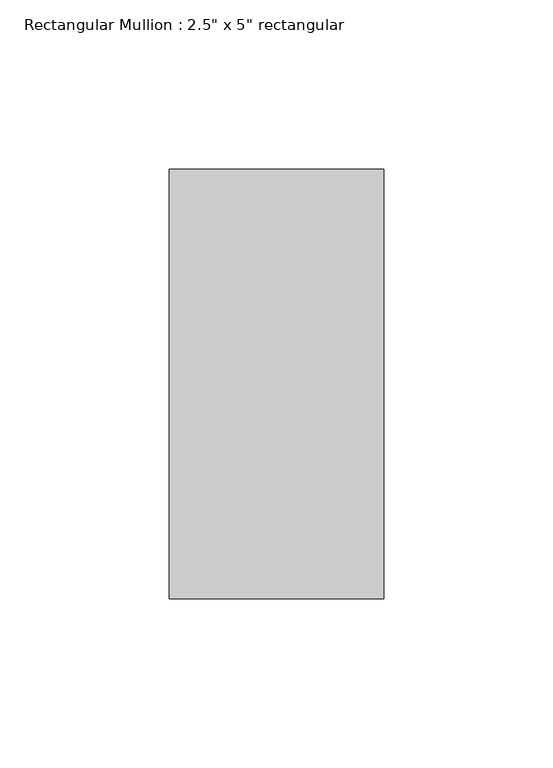
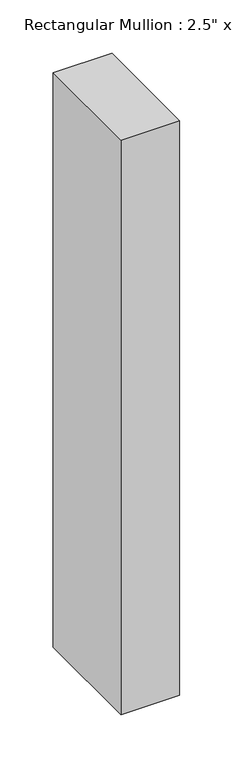
"""IFC4 building model written with IfcOpenShell, lengths in millimetres: member geometry."""

from ifc_helpers import new_model, si_unit, frame, origin, place, context, project, spatial, polyline, outline, extrude, source, transform, mapped, element, save


def member_1723abb6(model_context):
    return source(origin(), model_context, "Body", "SweptSolid", [
        extrude(outline(polyline([(0.0, 63.5), (0.0, -63.5), (-63.5, -63.5), (-63.5, 63.5), (0.0, 63.5)])), frame((0.0, 0.0, -657.1098201), z_axis=(0.0, 0.0, 1.0), x_axis=(1.0, 0.0, 0.0)), (0.0, 0.0, 1.0), 657.1098201),
    ])


if __name__ == "__main__":
    model = new_model("IFC4")
    model_context = context("Model", 3, world=origin())
    ifc_project = project(units=[si_unit("LENGTHUNIT", "METRE", prefix="MILLI")], contexts=[model_context])
    site = spatial("IfcSite", under=ifc_project)
    building = spatial("IfcBuilding", under=site)
    placement = place(None, origin())
    member_shape = member_1723abb6(model_context)
    element("IfcMember", 1, ObjectType="Rectangular Mullion : 2.5\" x 5\" rectangular", at=placement, inside=building, context=model_context, shape_type="MappedRepresentation", body=[
        mapped(member_shape, transform((0.0, 0.0, 0.0), x_axis=(1.0, 0.0, 0.0), y_axis=(0.0, 1.0, 0.0), z_axis=(0.0, 0.0, 1.0))),
    ])
    save(model, "model.ifc")

# Revit data of these elements
# Type "Rectangular Mullion : 2.5\" x 5\" rectangular"
#   built-in parameter 1007304 = 0.416667 (stored number, unit not read)
#   built-in parameter 1007301 = 0.104167 (stored number, unit not read)
#   built-in parameter 1007300 = 0.104167 (stored number, unit not read)
# Element 1 (IfcMember, "Rectangular Mullion : 2.5\" x 5\" rectangular")
#   Materials on its faces: "Aluminum"
# Materials
#   "Aluminum": class "Metal", colour RGB 247 247 247, transparency 0, Description = "Aluminum 6061", Cost = 0
